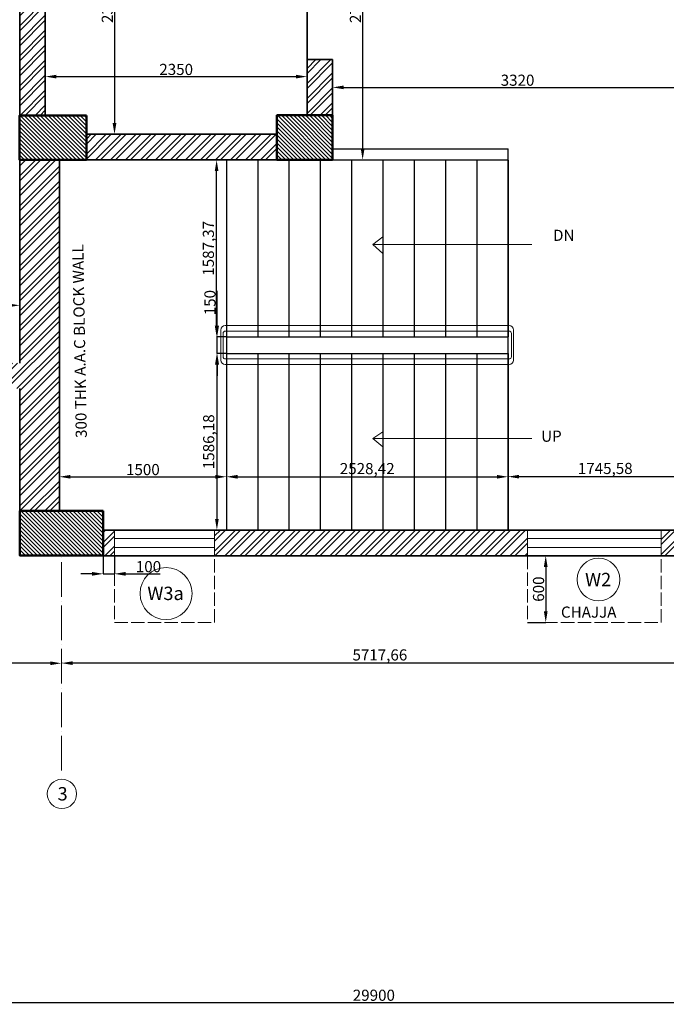
# Model space of a CAD drawing. Units: millimetres. Extents: x -3326 to 29338, y -16792 to 6002.
# Tile 6 of 21: x 11152 to 16958, y -16792 to -7951. Entities that reach past the tile are written whole.
import ezdxf

# ---------------------------------------------------------------- set-up
doc = ezdxf.new("R2010")
doc.units = ezdxf.units.MM
doc.header["$PDMODE"] = 35
doc.header["$PDSIZE"] = 5
doc.linetypes.add('ACAD_ISO02W100', pattern=[15, 12, -3])
doc.linetypes.add('ACAD_ISO04W100', pattern=[30, 24, -3, 0, -3])
for name, color, linetype, lineweight in [('A-ANNO-DIMS', 2, 'Continuous', 13), ('A-ANNO-SYMB', 7, 'Continuous', 18), ('A-COLS', 1, 'Continuous', 50), ('A-COLS-PATT', 251, 'Continuous', 13), ('A-FLOR-RAIL', 8, 'Continuous', 20), ('A-FLOR-STRS', 7, 'Continuous', 25), ('A-GLAZ', 4, 'Continuous', 18), ('A-GRID', 8, 'ACAD_ISO04W100', 13), ('A-GRID-IDEN', 7, 'Continuous', 18), ('A-ROOF-OVHD', 8, 'ACAD_ISO02W100', 13), ('A-WALL', 7, 'Continuous', 35), ('A-WALL-PATT', 252, 'Continuous', 13), ('txt', 7, 'Continuous', 18)]:
    doc.layers.add(name, color=color, linetype=linetype, lineweight=lineweight)
doc.styles.get("Standard").update_dxf_attribs({"font": 'arial.ttf'})
doc.dimstyles.new('ISO-25', dxfattribs={"dimtxt": 100, "dimasz": 100, "dimexe": 1.25, "dimexo": 0.625, "dimtad": 1, "dimtxsty": 'Standard', "dimcen": 2.5, "dimadec": 0, "dimazin": 0, "dimtfac": 1, "dimtmove": 0, "dimatfit": 3, "dimfxl": 1, "dimarcsym": 0})

# ---------------------------------------------------------------- blocks, each defined once
blk = doc.blocks.new('*D36')
at = {"layer": 'A-ANNO-DIMS', "color": 0, "lineweight": -2, "transparency": 16777216}
for p, q in [((11508.3, -11826.3), (11508.3, -12056.7)), ((13008.3, -11826.3), (13008.3, -12056.7)), ((11608.3, -12055.4), (12908.3, -12055.4))]:
    blk.add_line(p, q, dxfattribs=at)
at = {"layer": 'A-ANNO-DIMS', "color": 0, "transparency": 16777216}
for points in [[(11608.3, -12038.7), (11608.3, -12072.1), (11508.3, -12055.4)], [(12908.3, -12038.7), (12908.3, -12072.1), (13008.3, -12055.4)]]:
    blk.add_solid(points, dxfattribs=at)
at = {"layer": 'Defpoints', "color": 0, "transparency": 16777216}
for p in [(11508.3, -11825.7), (13008.3, -11825.7), (13008.3, -12055.4)]:
    blk.add_point(p, dxfattribs=at)
at = {"layer": 'A-ANNO-DIMS', "color": 0, "transparency": 16777216, "insert": (12258.3, -12003.7), "char_height": 100, "attachment_point": 5}
blk.add_mtext('1500', dxfattribs=at)
blk = doc.blocks.new('*D37')
at = {"layer": 'A-ANNO-DIMS', "color": 0, "lineweight": -2, "transparency": 16777216}
for p, q in [((13008.3, -12054.8), (13008.3, -12054.2)), ((13108.3, -12055.4), (15436.7, -12055.4)), ((15536.7, -12054.8), (15536.7, -12054.2))]:
    blk.add_line(p, q, dxfattribs=at)
at = {"layer": 'A-ANNO-DIMS', "color": 0, "transparency": 16777216}
for points in [[(13108.3, -12038.7), (13108.3, -12072.1), (13008.3, -12055.4)], [(15436.7, -12038.7), (15436.7, -12072.1), (15536.7, -12055.4)]]:
    blk.add_solid(points, dxfattribs=at)
at = {"layer": 'Defpoints', "color": 0, "transparency": 16777216}
for p in [(13008.3, -12055.4), (15536.7, -12055.4), (15536.7, -12055.4)]:
    blk.add_point(p, dxfattribs=at)
at = {"layer": 'A-ANNO-DIMS', "color": 0, "transparency": 16777216, "insert": (14272.5, -11994.7), "char_height": 100, "attachment_point": 5}
blk.add_mtext('2528,42', dxfattribs=at)
blk = doc.blocks.new('*D38')
at = {"layer": 'A-ANNO-DIMS', "color": 0, "lineweight": -2, "transparency": 16777216}
for p, q in [((15536.7, -12053.5), (15536.7, -12052.9)), ((15636.7, -12054.2), (17182.3, -12054.2)), ((17282.3, -12053.5), (17282.3, -12052.9))]:
    blk.add_line(p, q, dxfattribs=at)
at = {"layer": 'A-ANNO-DIMS', "color": 0, "transparency": 16777216}
for points in [[(15636.7, -12037.5), (15636.7, -12070.8), (15536.7, -12054.2)], [(17182.3, -12037.5), (17182.3, -12070.8), (17282.3, -12054.2)]]:
    blk.add_solid(points, dxfattribs=at)
at = {"layer": 'Defpoints', "color": 0, "transparency": 16777216}
for p in [(15536.7, -12054.2), (17282.3, -12054.2), (17282.3, -12054.2)]:
    blk.add_point(p, dxfattribs=at)
at = {"layer": 'A-ANNO-DIMS', "color": 0, "transparency": 16777216, "insert": (16409.5, -11993.4), "char_height": 100, "attachment_point": 5}
blk.add_mtext('1745,58', dxfattribs=at)
blk = doc.blocks.new('*D39')
at = {"layer": 'A-ANNO-DIMS', "color": 0, "lineweight": -2, "transparency": 16777216}
for p, q in [((13007.7, -10947.8), (12921.6, -10947.8)), ((12922.8, -11047.8), (12922.8, -12434)), ((13007.7, -12534), (12921.6, -12534))]:
    blk.add_line(p, q, dxfattribs=at)
at = {"layer": 'A-ANNO-DIMS', "color": 0, "transparency": 16777216}
for points in [[(12906.1, -11047.8), (12939.5, -11047.8), (12922.8, -10947.8)], [(12906.1, -12434), (12939.5, -12434), (12922.8, -12534)]]:
    blk.add_solid(points, dxfattribs=at)
at = {"layer": 'Defpoints', "color": 0, "transparency": 16777216}
for p in [(13008.3, -10947.8), (12922.8, -12534), (13008.3, -12534)]:
    blk.add_point(p, dxfattribs=at)
at = {"layer": 'A-ANNO-DIMS', "color": 0, "transparency": 16777216, "insert": (12862.1, -11740.9), "char_height": 100, "attachment_point": 5, "rotation": 90}
blk.add_mtext('1586,18', dxfattribs=at)
blk = doc.blocks.new('*D40')
at = {"layer": 'A-ANNO-DIMS', "color": 0, "lineweight": -2, "transparency": 16777216}
for p, q in [((12925.3, -10697.8), (12925.3, -10385.3)), ((13007.7, -10797.8), (12924, -10797.8)), ((12925.3, -10947.8), (12925.3, -10797.8)), ((13007.7, -10947.8), (12924, -10947.8)), ((12925.3, -11047.8), (12925.3, -11147.8))]:
    blk.add_line(p, q, dxfattribs=at)
at = {"layer": 'A-ANNO-DIMS', "color": 0, "transparency": 16777216}
for points in [[(12908.6, -10697.8), (12941.9, -10697.8), (12925.3, -10797.8)], [(12908.6, -11047.8), (12941.9, -11047.8), (12925.3, -10947.8)]]:
    blk.add_solid(points, dxfattribs=at)
at = {"layer": 'Defpoints', "color": 0, "transparency": 16777216}
for p in [(12925.3, -10797.8), (13008.3, -10797.8), (13008.3, -10947.8)]:
    blk.add_point(p, dxfattribs=at)
at = {"layer": 'A-ANNO-DIMS', "color": 0, "transparency": 16777216, "insert": (12873.6, -10491.6), "char_height": 100, "attachment_point": 5, "rotation": 90}
blk.add_mtext('150', dxfattribs=at)
blk = doc.blocks.new('*D41')
at = {"layer": 'A-ANNO-DIMS', "color": 0, "lineweight": -2, "transparency": 16777216}
for p, q in [((13007.7, -9210.4), (12919, -9210.4)), ((12920.3, -10697.8), (12920.3, -9310.4)), ((13007.7, -10797.8), (12919, -10797.8))]:
    blk.add_line(p, q, dxfattribs=at)
at = {"layer": 'A-ANNO-DIMS', "color": 0, "transparency": 16777216}
for points in [[(12903.6, -9310.4), (12936.9, -9310.4), (12920.3, -9210.4)], [(12903.6, -10697.8), (12936.9, -10697.8), (12920.3, -10797.8)]]:
    blk.add_solid(points, dxfattribs=at)
at = {"layer": 'Defpoints', "color": 0, "transparency": 16777216}
for p in [(12920.3, -9210.4), (13008.3, -9210.4), (13008.3, -10797.8)]:
    blk.add_point(p, dxfattribs=at)
at = {"layer": 'A-ANNO-DIMS', "color": 0, "transparency": 16777216, "insert": (12859.5, -10004.1), "char_height": 100, "attachment_point": 5, "rotation": 90}
blk.add_mtext('1587,37', dxfattribs=at)
blk = doc.blocks.new('*D42')
at = {"layer": 'A-ANNO-DIMS', "color": 0, "lineweight": -2, "transparency": 16777216}
for p, q in [((15712.9, -12764), (15876.6, -12764)), ((15875.3, -12864), (15875.3, -13264)), ((15712.9, -13364), (15876.6, -13364))]:
    blk.add_line(p, q, dxfattribs=at)
at = {"layer": 'A-ANNO-DIMS', "color": 0, "transparency": 16777216}
for points in [[(15858.7, -12864), (15892, -12864), (15875.3, -12764)], [(15858.7, -13264), (15892, -13264), (15875.3, -13364)]]:
    blk.add_solid(points, dxfattribs=at)
at = {"layer": 'Defpoints', "color": 0, "transparency": 16777216}
for p in [(15712.3, -12764), (15712.3, -13364), (15875.3, -13364)]:
    blk.add_point(p, dxfattribs=at)
at = {"layer": 'A-ANNO-DIMS', "color": 0, "transparency": 16777216, "insert": (15823.7, -13064), "char_height": 100, "attachment_point": 5, "rotation": 90}
blk.add_mtext('600', dxfattribs=at)
blk = doc.blocks.new('*D43')
at = {"layer": 'A-ANNO-DIMS', "color": 0, "lineweight": -2, "transparency": 16777216}
for p, q in [((11902.3, -12764.6), (11902.3, -12927.9)), ((12002.3, -12764.6), (12002.3, -12927.9)), ((11802.3, -12926.7), (11702.3, -12926.7)), ((11902.3, -12926.7), (12002.3, -12926.7)), ((12102.3, -12926.7), (12414.7, -12926.7))]:
    blk.add_line(p, q, dxfattribs=at)
at = {"layer": 'A-ANNO-DIMS', "color": 0, "transparency": 16777216}
for points in [[(11802.3, -12910), (11802.3, -12943.3), (11902.3, -12926.7)], [(12102.3, -12910), (12102.3, -12943.3), (12002.3, -12926.7)]]:
    blk.add_solid(points, dxfattribs=at)
at = {"layer": 'Defpoints', "color": 0, "transparency": 16777216}
for p in [(11902.3, -12764), (12002.3, -12764), (12002.3, -12926.7)]:
    blk.add_point(p, dxfattribs=at)
at = {"layer": 'A-ANNO-DIMS', "color": 0, "transparency": 16777216, "insert": (12308.5, -12875), "char_height": 100, "attachment_point": 5}
blk.add_mtext('100', dxfattribs=at)
blk = doc.blocks.new('*D45')
at = {"layer": 'A-ANNO-DIMS', "color": 0, "lineweight": -2, "transparency": 16777216}
for p, q in [((11382.3, -8461.9), (11382.3, -8461.3)), ((11482.3, -8462.5), (13632.3, -8462.5)), ((13732.3, -8461.9), (13732.3, -8461.3))]:
    blk.add_line(p, q, dxfattribs=at)
at = {"layer": 'A-ANNO-DIMS', "color": 0, "transparency": 16777216}
for points in [[(11482.3, -8445.9), (11482.3, -8479.2), (11382.3, -8462.5)], [(13632.3, -8445.9), (13632.3, -8479.2), (13732.3, -8462.5)]]:
    blk.add_solid(points, dxfattribs=at)
at = {"layer": 'Defpoints', "color": 0, "transparency": 16777216}
for p in [(11382.3, -8462.5), (13732.3, -8462.5), (13732.3, -8462.5)]:
    blk.add_point(p, dxfattribs=at)
at = {"layer": 'A-ANNO-DIMS', "color": 0, "transparency": 16777216, "insert": (12557.3, -8410.8), "char_height": 100, "attachment_point": 5}
blk.add_mtext('2350', dxfattribs=at)
blk = doc.blocks.new('*D46')
at = {"layer": 'A-ANNO-DIMS', "color": 0, "lineweight": -2, "transparency": 16777216}
for p, q in [((11797.4, -6680.4), (12004.9, -6680.4)), ((12003.7, -6780.4), (12003.7, -8880.4)), ((11797.4, -8980.4), (12004.9, -8980.4))]:
    blk.add_line(p, q, dxfattribs=at)
at = {"layer": 'A-ANNO-DIMS', "color": 0, "transparency": 16777216}
for points in [[(11987, -6780.4), (12020.4, -6780.4), (12003.7, -6680.4)], [(11987, -8880.4), (12020.4, -8880.4), (12003.7, -8980.4)]]:
    blk.add_solid(points, dxfattribs=at)
at = {"layer": 'Defpoints', "color": 0, "transparency": 16777216}
for p in [(11796.7, -6680.4), (11796.7, -8980.4), (12003.7, -8980.4)]:
    blk.add_point(p, dxfattribs=at)
at = {"layer": 'A-ANNO-DIMS', "color": 0, "transparency": 16777216, "insert": (11952, -7830.4), "char_height": 100, "attachment_point": 5, "rotation": 90}
blk.add_mtext('2300', dxfattribs=at)
blk = doc.blocks.new('*D47')
at = {"layer": 'A-ANNO-DIMS', "color": 0, "lineweight": -2, "transparency": 16777216}
for p, q in [((13962.9, -6450.4), (14232.6, -6450.4)), ((14231.3, -6550.4), (14231.3, -9110.4)), ((13962.9, -9210.4), (14232.6, -9210.4))]:
    blk.add_line(p, q, dxfattribs=at)
at = {"layer": 'A-ANNO-DIMS', "color": 0, "transparency": 16777216}
for points in [[(14214.7, -6550.4), (14248, -6550.4), (14231.3, -6450.4)], [(14214.7, -9110.4), (14248, -9110.4), (14231.3, -9210.4)]]:
    blk.add_solid(points, dxfattribs=at)
at = {"layer": 'Defpoints', "color": 0, "transparency": 16777216}
for p in [(13962.3, -6450.4), (13962.3, -9210.4), (14231.3, -9210.4)]:
    blk.add_point(p, dxfattribs=at)
at = {"layer": 'A-ANNO-DIMS', "color": 0, "transparency": 16777216, "insert": (14179.6, -7830.4), "char_height": 100, "attachment_point": 5, "rotation": 90}
blk.add_mtext('2760', dxfattribs=at)
blk = doc.blocks.new('*D48')
at = {"layer": 'A-ANNO-DIMS', "color": 0, "lineweight": -2, "transparency": 16777216}
for p, q in [((13962.3, -8558.9), (13962.3, -8558.2)), ((14062.3, -8559.5), (17182.3, -8559.5)), ((17282.3, -8558.9), (17282.3, -8558.2))]:
    blk.add_line(p, q, dxfattribs=at)
at = {"layer": 'A-ANNO-DIMS', "color": 0, "transparency": 16777216}
for points in [[(14062.3, -8542.8), (14062.3, -8576.1), (13962.3, -8559.5)], [(17182.3, -8542.8), (17182.3, -8576.1), (17282.3, -8559.5)]]:
    blk.add_solid(points, dxfattribs=at)
at = {"layer": 'Defpoints', "color": 0, "transparency": 16777216}
for p in [(13962.3, -8559.5), (17282.3, -8559.5), (17282.3, -8559.5)]:
    blk.add_point(p, dxfattribs=at)
at = {"layer": 'A-ANNO-DIMS', "color": 0, "transparency": 16777216, "insert": (15622.3, -8507.8), "char_height": 100, "attachment_point": 5}
blk.add_mtext('3320', dxfattribs=at)
blk = doc.blocks.new('*D58')
at = {"layer": 'A-ANNO-DIMS', "color": 0, "lineweight": -2, "transparency": 16777216}
for p, q in [((7302.3, -10583), (7302.3, -10514.7)), ((7402.3, -10515.9), (11052.3, -10515.9)), ((11152.3, -10583), (11152.3, -10514.7))]:
    blk.add_line(p, q, dxfattribs=at)
at = {"layer": 'A-ANNO-DIMS', "color": 0, "transparency": 16777216}
for points in [[(7402.3, -10499.2), (7402.3, -10532.6), (7302.3, -10515.9)], [(11052.3, -10499.2), (11052.3, -10532.6), (11152.3, -10515.9)]]:
    blk.add_solid(points, dxfattribs=at)
at = {"layer": 'Defpoints', "color": 0, "transparency": 16777216}
for p in [(11152.3, -10515.9), (7302.3, -10583.6), (11152.3, -10583.6)]:
    blk.add_point(p, dxfattribs=at)
at = {"layer": 'A-ANNO-DIMS', "color": 0, "transparency": 16777216, "insert": (9227.3, -10464.2), "char_height": 100, "attachment_point": 5}
blk.add_mtext('3850', dxfattribs=at)
blk = doc.blocks.new('*D159')
at = {"layer": 'A-ANNO-DIMS', "color": 0, "lineweight": -2, "transparency": 16777216}
for p, q in [((11527.3, -13721), (11527.3, -13729.7)), ((17145, -13728.4), (11627.3, -13728.4)), ((17245, -13721), (17245, -13729.7))]:
    blk.add_line(p, q, dxfattribs=at)
at = {"layer": 'A-ANNO-DIMS', "color": 0, "transparency": 16777216}
for points in [[(11627.3, -13711.8), (11627.3, -13745.1), (11527.3, -13728.4)], [(17145, -13711.8), (17145, -13745.1), (17245, -13728.4)]]:
    blk.add_solid(points, dxfattribs=at)
at = {"layer": 'Defpoints', "color": 0, "transparency": 16777216}
for p in [(11527.3, -13720.4), (11527.3, -13728.4), (17245, -13720.4)]:
    blk.add_point(p, dxfattribs=at)
at = {"layer": 'A-ANNO-DIMS', "color": 0, "transparency": 16777216, "insert": (14386.1, -13667.7), "char_height": 100, "attachment_point": 5}
blk.add_mtext('5717,66', dxfattribs=at)
blk = doc.blocks.new('*D160')
at = {"layer": 'A-ANNO-DIMS', "color": 0, "lineweight": -2, "transparency": 16777216}
for p, q in [((5390, -13729), (5390, -13728.4)), ((11427.3, -13729.7), (5490, -13729.7)), ((11527.3, -13729), (11527.3, -13728.4))]:
    blk.add_line(p, q, dxfattribs=at)
at = {"layer": 'A-ANNO-DIMS', "color": 0, "transparency": 16777216}
for points in [[(5490, -13713), (5490, -13746.3), (5390, -13729.7)], [(11427.3, -13713), (11427.3, -13746.3), (11527.3, -13729.7)]]:
    blk.add_solid(points, dxfattribs=at)
at = {"layer": 'Defpoints', "color": 0, "transparency": 16777216}
for p in [(5390, -13729.7), (5390, -13729.7), (11527.3, -13729.7)]:
    blk.add_point(p, dxfattribs=at)
at = {"layer": 'A-ANNO-DIMS', "color": 0, "transparency": 16777216, "insert": (8458.6, -13668.9), "char_height": 100, "attachment_point": 5}
blk.add_mtext('6137,34', dxfattribs=at)
blk = doc.blocks.new('*D235')
at = {"layer": 'A-ANNO-DIMS', "color": 0, "lineweight": -2, "transparency": 16777216}
for p, q in [((-617.7, -12764.6), (-617.7, -16776.1)), ((29282.3, -12764.6), (29282.3, -16776.1)), ((-517.7, -16774.9), (29182.3, -16774.9))]:
    blk.add_line(p, q, dxfattribs=at)
at = {"layer": 'A-ANNO-DIMS', "color": 0, "transparency": 16777216}
for points in [[(-517.7, -16758.2), (-517.7, -16791.6), (-617.7, -16774.9)], [(29182.3, -16758.2), (29182.3, -16791.6), (29282.3, -16774.9)]]:
    blk.add_solid(points, dxfattribs=at)
at = {"layer": 'Defpoints', "color": 0, "transparency": 16777216}
for p in [(-617.7, -12764), (29282.3, -12764), (29282.3, -16774.9)]:
    blk.add_point(p, dxfattribs=at)
at = {"layer": 'A-ANNO-DIMS', "color": 0, "transparency": 16777216, "insert": (14332.3, -16723.2), "char_height": 100, "attachment_point": 5}
blk.add_mtext('29900', dxfattribs=at)

msp = doc.modelspace()

# ---------------------------------------------------------------- hatches: boundary and pattern name
at = {"layer": 'A-COLS-PATT'}
h = msp.add_hatch(dxfattribs=at)
h.set_pattern_fill('ANSI31', color=256, scale=8, angle=-90)
h.set_pattern_definition([(315, (18358.179, 32910.899), (17.960512, 17.960512), [])])
h.paths.add_polyline_path([(11151.174, -8810.401), (11151.174, -9210.401), (11751.174, -9210.401), (11751.174, -8810.401)])
h = msp.add_hatch(dxfattribs=at)
h.set_pattern_fill('ANSI31', color=256, scale=8, angle=-90)
h.set_pattern_definition([(315, (19175.939, 35806.228), (17.960512, 17.960512), [])])
h.paths.add_polyline_path([(13962.301, -8809.482), (13462.301, -8809.482), (13462.301, -9209.482), (13962.301, -9209.482)])
h = msp.add_hatch(dxfattribs=at)
h.set_pattern_fill('ANSI31', color=256, scale=8, angle=-90)
h.set_pattern_definition([(315, (22071.838, 29677.046), (17.960512, 17.960512), [])])
h.paths.add_polyline_path([(11902.301, -12761.585), (11902.301, -12361.585), (11152.301, -12361.585), (11152.301, -12761.585)])
at = {"layer": 'A-WALL-PATT'}
h = msp.add_hatch(dxfattribs=at)
h.set_pattern_fill('ANSI32', color=256, scale=10)
h.set_pattern_definition([(45, (-10476.65, 1e-12), (-67.35192, 67.35192), []), (45, (-10431.74, 1e-12), (-67.35192, 67.35192), [])])
h.paths.add_polyline_path([(12212.301, -1983.952), (11640.861, -1983.952), (11640.861, -2213.952), (12212.301, -2213.952)])
h.paths.add_polyline_path([(14712.301, -1983.952), (14012.301, -1983.952), (14012.301, -2213.952), (14712.301, -2213.952)])
h.paths.add_polyline_path([(17012.301, -1983.952), (16512.301, -1983.952), (16512.301, -2213.952), (17012.301, -2213.952)])
h.paths.add_polyline_path([(11382.301, -2383.952), (11040.861, -2383.952), (7302.301, -2383.952), (7302.301, -1935.766), (7217.026, -1935.766), (7202.301, -1933.952), (7202.301, -2483.952), (7302.301, -2483.952), (11152.301, -2483.952), (11152.301, -2833.952), (11283.549, -2833.952), (11283.549, -2830.395), (11363.875, -2830.395), (11382.301, -2833.952)])
h.paths.add_polyline_path([(11382.301, -3733.952), (11363.875, -3733.952), (11363.875, -3734.058), (11283.549, -3734.058), (11152.301, -3733.952), (11152.301, -6450.401), (11382.301, -6450.401)])
h.paths.add_polyline_path([(13462.301, -6450.401), (12606.738, -6450.401), (11382.301, -6450.401), (11382.301, -6680.401), (12606.738, -6680.401), (13462.301, -6680.401)])
h.paths.add_polyline_path([(11382.301, -7050.401), (11152.301, -7050.401), (11152.301, -8810.401), (11382.301, -8810.401)])
h.paths.add_polyline_path([(13462.301, -8980.401), (11751.174, -8980.401), (11751.174, -9210.401), (13462.301, -9210.401)])
h.paths.add_polyline_path([(13962.301, -6850.401), (13732.301, -6850.401), (13732.301, -7350.401), (13962.301, -7350.401)])
h.paths.add_polyline_path([(13962.301, -8309.482), (13732.301, -8309.482), (13732.301, -8809.482), (13962.301, -8809.482)])
h.paths.add_polyline_path([(15712.301, -12533.952), (12902.301, -12533.952), (12902.301, -12763.952), (15712.301, -12763.952)])
h.paths.add_polyline_path([(11508.301, -9211.585), (11382.301, -9211.585), (11152.301, -9211.585), (11152.301, -11033.952), (10952.301, -11033.952), (10952.301, -11263.952), (11152.301, -11263.952), (11152.301, -12361.585), (11508.301, -12361.585)])
h.paths.add_polyline_path([(12002.301, -12533.952), (11902.301, -12533.952), (11902.301, -12761.585), (11152.301, -12761.585), (11152.301, -12763.952), (11902.301, -12763.952), (12002.301, -12763.952)])
h.paths.add_polyline_path([(17112.301, -12533.952), (16912.301, -12533.952), (16912.301, -12763.952), (17112.301, -12763.952)])
h.paths.add_polyline_path([(11382.301, 3596.048), (11152.301, 3596.048), (11152.301, 2096.048), (11382.301, 2096.048)])
h.paths.add_polyline_path([(11382.301, 1496.048), (11152.301, 1496.048), (11152.301, -1983.952), (11382.301, -1983.952)])

# ---------------------------------------------------------------- linework, layer by layer
at = {"layer": 'A-ANNO-SYMB'}
for p, q in [((14324.08, -9969.776), (14412.977, -9901.24)), ((15751.74, -9969.776), (14324.08, -9969.776)), ((14324.08, -9969.776), (14412.977, -10050.515)), ((14324.08, -11710.729), (14412.977, -11652.585)), ((15751.74, -11710.729), (14324.08, -11710.729)), ((14324.08, -11710.729), (14399.198, -11710.729)), ((14324.08, -11710.729), (14412.977, -11785.776))]:
    msp.add_line(p, q, dxfattribs=at)
for centre, radius in [((16348.884, -12978.301), 191.81), ((12466.49, -13103.418), 233.823)]:
    msp.add_circle(centre, radius, dxfattribs=at)
at = {"layer": 'A-COLS'}
for points in [[(11751.174, -8810.401), (11751.174, -9210.401), (11151.174, -9210.401), (11151.174, -8810.401)], [(13962.301, -8809.482), (13962.301, -9209.482), (13462.301, -9209.482), (13462.301, -8809.482)], [(11902.301, -12361.585), (11902.301, -12761.585), (11152.301, -12761.585), (11152.301, -12361.585)]]:
    msp.add_lwpolyline(points, close=True, dxfattribs=at)
at = {"layer": 'A-FLOR-RAIL'}
for p, q in [((12958.301, -10737.769), (12958.301, -11007.769)), ((12978.301, -10977.769), (12978.301, -10767.769)), ((13008.301, -10697.769), (12998.301, -10697.769)), ((13008.301, -10747.769), (12998.301, -10747.769)), ((13008.301, -10697.769), (15536.718, -10697.769)), ((13008.301, -10747.769), (15536.718, -10747.769)), ((15536.718, -10697.769), (15546.718, -10697.769)), ((15536.718, -10747.769), (15546.718, -10747.769)), ((15566.718, -10977.769), (15566.718, -10767.769)), ((15586.718, -10737.769), (15586.718, -11007.769)), ((13008.301, -10997.769), (12998.301, -10997.769)), ((13008.301, -11047.769), (12998.301, -11047.769)), ((13008.301, -10997.769), (15536.718, -10997.769)), ((13008.301, -11047.769), (15536.718, -11047.769)), ((15536.718, -10997.769), (15546.718, -10997.769)), ((15536.718, -11047.769), (15546.718, -11047.769))]:
    msp.add_line(p, q, dxfattribs=at)
for centre, radius, start, end in [((12998.301, -10737.769), 40, 90, 180), ((12998.301, -10767.769), 20, 90, 180), ((15546.718, -10737.769), 40, 360, 90), ((15546.718, -10767.769), 20, 0, 90), ((12998.301, -11007.769), 40, 180, 270), ((12998.301, -10977.769), 20, 180, 270), ((15546.718, -10977.769), 20, 270, 0), ((15546.718, -11007.769), 40, 270, 360)]:
    msp.add_arc(centre, radius, start, end, dxfattribs=at)
at = {"layer": 'A-FLOR-STRS'}
for p, q in [((13962.301, -9110.401), (15536.718, -9110.401)), ((15536.718, -9210.401), (15536.718, -9110.401)), ((13008.301, -9211.585), (13008.301, -10797.769)), ((13289.236, -9211.585), (13289.236, -10797.769)), ((13570.171, -9211.585), (13570.171, -10797.769)), ((13851.106, -9211.585), (13851.106, -10797.769)), ((13962.301, -9210.401), (15536.718, -9210.401)), ((14132.042, -9211.585), (14132.042, -10797.769)), ((14412.977, -9211.585), (14412.977, -10797.769)), ((14693.912, -9211.585), (14693.912, -10797.769)), ((14974.847, -9211.585), (14974.847, -10797.769)), ((15255.782, -9211.585), (15255.782, -10797.769)), ((15536.718, -12533.952), (15536.718, -9210.401)), ((15536.718, -9211.585), (15536.718, -10797.769)), ((13008.301, -10797.769), (15536.718, -10797.769)), ((13008.301, -10797.769), (13008.301, -10947.769)), ((13008.301, -10947.769), (15536.718, -10947.769)), ((13008.301, -10947.769), (13008.301, -12533.952)), ((13289.236, -10947.769), (13289.236, -12533.952)), ((13570.171, -10947.769), (13570.171, -12533.952)), ((13851.106, -10947.769), (13851.106, -12533.952)), ((14132.042, -10947.769), (14132.042, -12533.952)), ((14412.977, -10947.769), (14412.977, -12533.952)), ((14693.912, -10947.769), (14693.912, -12533.952)), ((14974.847, -10947.769), (14974.847, -12533.952)), ((15255.782, -10947.769), (15255.782, -12533.952)), ((15536.718, -10947.769), (15536.718, -12533.952))]:
    msp.add_line(p, q, dxfattribs=at)
at = {"layer": 'A-GLAZ'}
for p, q in [((12002.301, -12533.952), (12002.301, -12763.952)), ((12902.301, -12533.952), (12902.301, -12763.952)), ((15712.301, -12533.952), (15712.301, -12763.952)), ((16912.301, -12533.952), (16912.301, -12763.952)), ((12002.301, -12608.952), (12902.301, -12608.952)), ((15712.301, -12608.952), (16912.301, -12608.952)), ((12002.301, -12688.952), (12902.301, -12688.952)), ((15712.301, -12688.952), (16912.301, -12688.952))]:
    msp.add_line(p, q, dxfattribs=at)
at = {"layer": 'A-GRID', "ltscale": 13}
msp.add_line((11527.301, -14692.885), (11527.301, -12763.952), dxfattribs=at)
at = {"layer": 'A-GRID-IDEN'}
msp.add_circle((11531.532, -14902.678), 131.457, dxfattribs=at)
at = {"layer": 'A-ROOF-OVHD', "ltscale": 10}
for p, q in [((12002.301, -12763.952), (12002.301, -13363.952)), ((12902.301, -13363.952), (12902.301, -12763.952)), ((15712.301, -12763.952), (15712.301, -13363.952)), ((16912.301, -13363.952), (16912.301, -12763.952)), ((12002.301, -13363.952), (12902.301, -13363.952)), ((15712.301, -13363.952), (16912.301, -13363.952))]:
    msp.add_line(p, q, dxfattribs=at)
at = {"layer": 'A-WALL'}
for p, q in [((11382.301, -3733.952), (11382.301, -8810.401)), ((13732.301, -6850.401), (13732.301, -8809.482)), ((11152.301, -7050.401), (11152.301, -9211.585)), ((13962.301, -8309.482), (13732.301, -8309.482)), ((13962.301, -8309.482), (13962.301, -8809.482)), ((11751.174, -8980.401), (13462.301, -8980.401)), ((11152.301, -9211.585), (11382.301, -9211.585)), ((11152.301, -9211.585), (11152.301, -11033.952)), ((11382.301, -9211.585), (11508.301, -9211.585)), ((11508.301, -9211.585), (11508.301, -12361.585)), ((11751.174, -9210.401), (13962.301, -9210.401)), ((11152.301, -11263.952), (11152.301, -12763.952)), ((17112.301, -12533.952), (11902.301, -12533.952)), ((11902.301, -12763.952), (11152.301, -12763.952)), ((17112.301, -12763.952), (11902.301, -12763.952))]:
    msp.add_line(p, q, dxfattribs=at)

# ---------------------------------------------------------------- texts
at = {"layer": 'A-ANNO-SYMB', "attachment_point": 1}
for s, width, insert, char_height in [('DN', 671.12796, (15940.964, -9837.115), 100), ('UP', 184.89816, (15834, -11640.962), 100), ('W2', 253.35997, (16228.598, -12918.056), 120), ('W3a', 254.02762, (12298.727, -13042.108), 120)]:
    msp.add_mtext_dynamic_manual_height_columns(s, width=width, gutter_width=12.5, heights=[0], dxfattribs=dict(at, insert=insert, char_height=char_height))
at = {"layer": 'A-GRID-IDEN', "insert": (11492.242, -14841.368), "char_height": 120, "attachment_point": 1}
msp.add_mtext_dynamic_manual_height_columns('3', width=551.68587, gutter_width=12.5, heights=[0], dxfattribs=at)
at = {"layer": 'txt', "insert": (11655.66, -11707.557), "char_height": 100, "attachment_point": 1, "rotation": 91.0460749}
msp.add_mtext_dynamic_manual_height_columns('300 THK A.A.C BLOCK WALL', width=6222.68924, gutter_width=12.5, heights=[0], dxfattribs=at)
at = {"layer": 'txt', "insert": (16012.064, -13220.231), "char_height": 100, "attachment_point": 1}
msp.add_mtext_dynamic_manual_height_columns('CHAJJA', width=659.30637, gutter_width=12.5, heights=[0], dxfattribs=at)

# ---------------------------------------------------------------- dimensions: what is measured, and where the dimension line sits
at = {"layer": 'A-ANNO-DIMS'}
for base, p1, p2, picture, middle in [((14231.319, -9210.401), (13962.301, -6450.401), (13962.301, -9210.401), '*D47', (14179.637, -7830.401)), ((12003.695, -8980.401), (11796.744, -6680.401), (11796.744, -8980.401), '*D46', (11951.978, -7830.401)), ((12920.266, -9210.401), (13008.301, -10797.769), (13008.301, -9210.401), '*D41', (12859.546, -10004.085)), ((12925.257, -10797.769), (13008.301, -10947.769), (13008.301, -10797.769), '*D40', (12873.575, -10491.55)), ((12922.815, -12533.952), (13008.301, -10947.769), (13008.301, -12533.952), '*D39', (12862.095, -11740.86))]:
    dim = msp.add_linear_dim(base=base, p1=p1, p2=p2, angle=90, dimstyle='ISO-25', override={"dimclrd": 0, "dimclre": 0, "dimclrt": 0}, dxfattribs=at)
    dim.commit()
    dim.dimension.update_dxf_attribs({"geometry": picture, "text_midpoint": middle})
for base, p1, p2, override, picture, middle in [((13732.301, -8462.517), (11382.301, -8462.517), (13732.301, -8462.517), {"dimclrd": 0, "dimclre": 0, "dimclrt": 0}, '*D45', (12557.301, -8410.8)), ((17282.301, -8559.482), (13962.301, -8559.482), (17282.301, -8559.482), {"dimclrd": 0, "dimclre": 0, "dimclrt": 0}, '*D48', (15622.301, -8507.765)), ((11152.301, -10515.904), (7302.301, -10583.602), (11152.301, -10583.602), {"dimclrd": 0, "dimclre": 0, "dimclrt": 0}, '*D58', (9227.301, -10464.188)), ((13008.301, -12055.402), (11508.301, -11825.714), (13008.301, -11825.714), {"dimclrd": 0, "dimclre": 0, "dimclrt": 0}, '*D36', (12258.301, -12003.72)), ((15536.718, -12055.402), (13008.301, -12055.402), (15536.718, -12055.402), {"dimclrd": 0, "dimclre": 0, "dimclrt": 0}, '*D37', (14272.509, -11994.682)), ((17282.301, -12054.152), (15536.718, -12054.152), (17282.301, -12054.152), {"dimclrd": 0, "dimclre": 0, "dimclrt": 0}, '*D38', (16409.509, -11993.432)), ((29282.301, -16774.892), (-617.699, -12763.952), (29282.301, -12763.952), {"dimdec": 0, "dimlfac": 1, "dimrnd": 0, "dimzin": 0, "dimdsep": 46, "dimlunit": 2}, '*D235', (14332.301, -16723.21)), ((12002.301, -12926.663), (11902.301, -12763.952), (12002.301, -12763.952), {"dimclrd": 0, "dimclre": 0, "dimclrt": 0}, '*D43', (12308.519, -12874.981)), ((5389.9656, -13729.6686), (11527.3007, -13729.6686), (5389.9656, -13729.6686), {"dimclrd": 0, "dimclre": 0, "dimclrt": 0}, '*D160', (8458.6331, -13668.9481)), ((11527.3007, -13728.4186), (17244.9656, -13720.4224), (11527.3007, -13720.4224), {"dimclrd": 0, "dimclre": 0, "dimclrt": 0}, '*D159', (14386.1331, -13667.6981))]:
    dim = msp.add_linear_dim(base=base, p1=p1, p2=p2, dimstyle='ISO-25', override=override, dxfattribs=at)
    dim.commit()
    dim.dimension.update_dxf_attribs({"geometry": picture, "text_midpoint": middle})
dim = msp.add_linear_dim(base=(15875.345, -13363.952), p1=(15712.301, -12763.952), p2=(15712.301, -13363.952), angle=90, dimstyle='ISO-25', override={"dimclrd": 0, "dimclre": 0, "dimclrt": 0}, dxfattribs=at)
dim.commit()
dim.dimension.update_dxf_attribs({"geometry": '*D42', "text_midpoint": (15875.345, -13063.952), "dimtype": 160})

doc.saveas('drawing.dxf')
